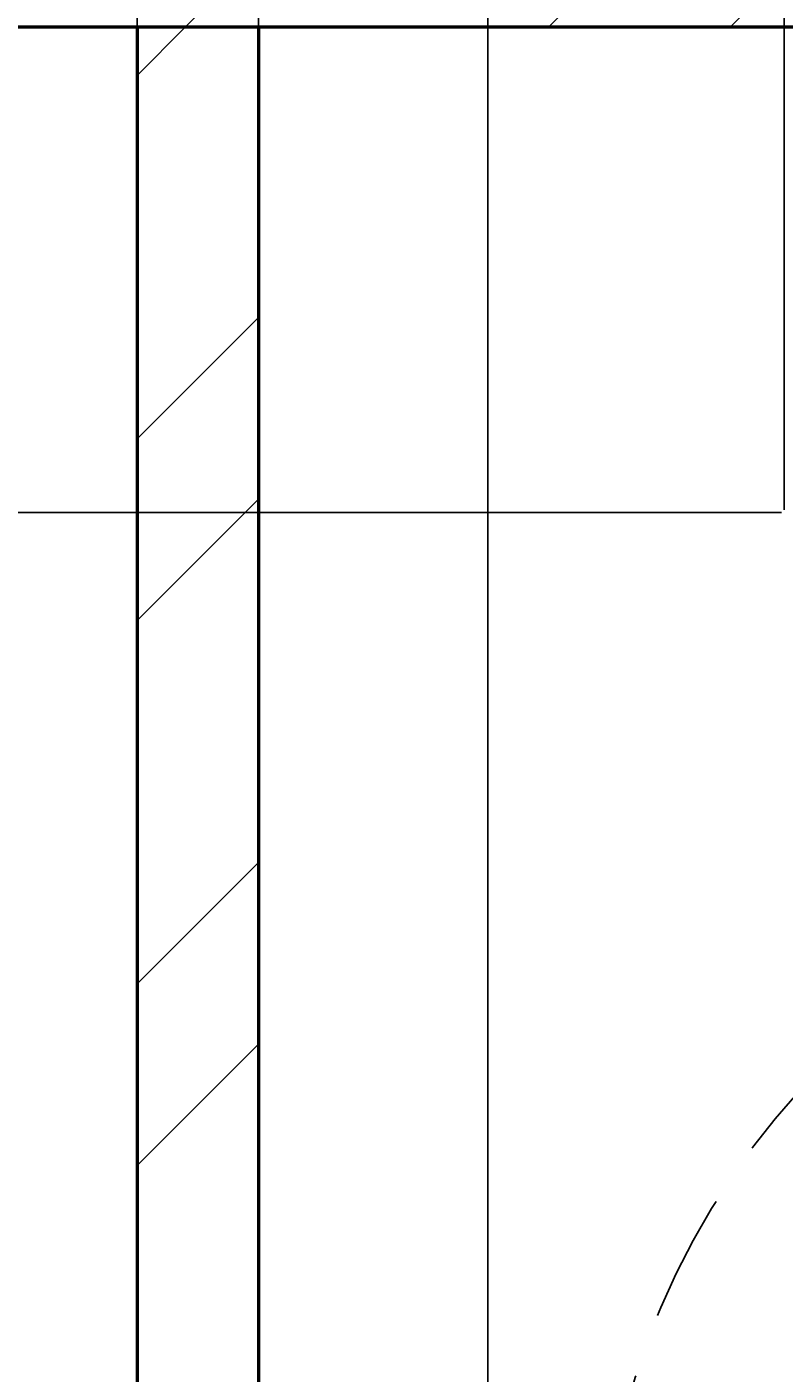
# Model space of a CAD drawing. Units: inches. Extents: x 2812 to 3051, y 1398 to 1659.
# Tile 53 of 65: x 2878 to 2896, y 1605 to 1638. Entities that reach past the tile are written whole.
import ezdxf

# ---------------------------------------------------------------- set-up
doc = ezdxf.new("R2010")
doc.units = ezdxf.units.IN
doc.linetypes.add('HIDDEN2', pattern=[4.7625, 3.175, -1.5875])
for name, color, linetype, lineweight in [('A-ANNO-DIMS', 2, 'Continuous', 18), ('S-CONC', 7, 'Continuous', 50), ('S-CONC-HIDN', 8, 'HIDDEN2', 25), ('S-CONC-PATT', 8, 'Continuous', 18)]:
    doc.layers.add(name, color=color, linetype=linetype, lineweight=lineweight)
doc.styles.get("Standard").update_dxf_attribs({"font": 'arial.ttf'})
doc.dimstyles.get("Standard").update_dxf_attribs({"dimtxt": 0.18, "dimasz": 0.18, "dimexe": 0.18, "dimexo": 0.0625, "dimgap": 0.09, "dimtad": 0, "dimtih": 1, "dimtoh": 1, "dimdec": 4, "dimzin": 0, "dimdsep": 46, "dimtxsty": 'Standard', "dimcen": 0.09, "dimadec": 0, "dimazin": 0, "dimtfac": 1, "dimtdec": 4, "dimtofl": 0, "dimtmove": 0, "dimatfit": 3, "dimfxl": 1, "dimtolj": 1, "dimtzin": 0, "dimarcsym": 0})

# ---------------------------------------------------------------- blocks, each defined once
blk = doc.blocks.new('*D17')
at = {"layer": 'A-ANNO-DIMS', "color": 0, "lineweight": -2, "transparency": 16777216}
for p, q in [((2883.385, 1637.882), (2883.385, 1659.35)), ((2896.385, 1625.882), (2896.385, 1659.35)), ((2883.565, 1659.17), (2889.674, 1659.17)), ((2896.205, 1659.17), (2890.095, 1659.17))]:
    blk.add_line(p, q, dxfattribs=at)
at = {"layer": 'A-ANNO-DIMS', "color": 0, "transparency": 16777216}
for points in [[(2883.565, 1659.2), (2883.565, 1659.14), (2883.385, 1659.17)], [(2896.205, 1659.2), (2896.205, 1659.14), (2896.385, 1659.17)]]:
    blk.add_solid(points, dxfattribs=at)
at = {"layer": 'Defpoints', "color": 0, "transparency": 16777216}
for p in [(2896.385, 1659.17), (2883.385, 1637.82), (2896.385, 1625.82)]:
    blk.add_point(p, dxfattribs=at)
at = {"layer": 'A-ANNO-DIMS', "color": 0, "transparency": 16777216, "insert": (2889.885, 1659.17), "char_height": 0.18, "attachment_point": 5}
blk.add_mtext('\\A1;13', dxfattribs=at)
blk = doc.blocks.new('*D18')
at = {"layer": 'A-ANNO-DIMS', "color": 0, "lineweight": -2, "transparency": 16777216}
for p, q in [((2896.385, 1625.882), (2896.385, 1659.35)), ((2905.385, 1625.882), (2905.385, 1659.35)), ((2896.565, 1659.17), (2900.736, 1659.17)), ((2905.205, 1659.17), (2901.034, 1659.17))]:
    blk.add_line(p, q, dxfattribs=at)
at = {"layer": 'A-ANNO-DIMS', "color": 0, "transparency": 16777216}
for points in [[(2896.565, 1659.2), (2896.565, 1659.14), (2896.385, 1659.17)], [(2905.205, 1659.2), (2905.205, 1659.14), (2905.385, 1659.17)]]:
    blk.add_solid(points, dxfattribs=at)
at = {"layer": 'Defpoints', "color": 0, "transparency": 16777216}
for p in [(2905.385, 1659.17), (2896.385, 1625.82), (2905.385, 1625.82)]:
    blk.add_point(p, dxfattribs=at)
at = {"layer": 'A-ANNO-DIMS', "color": 0, "transparency": 16777216, "insert": (2900.885, 1659.17), "char_height": 0.18, "attachment_point": 5}
blk.add_mtext('\\A1;9', dxfattribs=at)
blk = doc.blocks.new('*D38')
at = {"layer": 'A-ANNO-DIMS', "color": 0, "lineweight": -2, "transparency": 16777216}
for p, q in [((2896.322, 1625.82), (2811.806, 1625.82)), ((2811.986, 1625.64), (2811.986, 1612.5)), ((2811.986, 1599), (2811.986, 1612.14)), ((2910.679, 1598.82), (2811.806, 1598.82))]:
    blk.add_line(p, q, dxfattribs=at)
at = {"layer": 'A-ANNO-DIMS', "color": 0, "transparency": 16777216}
for points in [[(2811.956, 1625.64), (2812.016, 1625.64), (2811.986, 1625.82)], [(2811.956, 1599), (2812.016, 1599), (2811.986, 1598.82)]]:
    blk.add_solid(points, dxfattribs=at)
at = {"layer": 'Defpoints', "color": 0, "transparency": 16777216}
for p in [(2811.986, 1625.82), (2896.385, 1625.82), (2910.742, 1598.82)]:
    blk.add_point(p, dxfattribs=at)
at = {"layer": 'A-ANNO-DIMS', "color": 0, "transparency": 16777216, "insert": (2811.986, 1612.32), "char_height": 0.18, "attachment_point": 5}
blk.add_mtext('\\A1;27', dxfattribs=at)
blk = doc.blocks.new('*D39')
at = {"layer": 'A-ANNO-DIMS', "color": 0, "lineweight": -2, "transparency": 16777216}
for p, q in [((2883.322, 1637.82), (2811.806, 1637.82)), ((2811.986, 1637.64), (2811.986, 1632)), ((2811.986, 1626), (2811.986, 1631.64)), ((2896.322, 1625.82), (2811.806, 1625.82))]:
    blk.add_line(p, q, dxfattribs=at)
at = {"layer": 'A-ANNO-DIMS', "color": 0, "transparency": 16777216}
for points in [[(2811.956, 1637.64), (2812.016, 1637.64), (2811.986, 1637.82)], [(2811.956, 1626), (2812.016, 1626), (2811.986, 1625.82)]]:
    blk.add_solid(points, dxfattribs=at)
at = {"layer": 'Defpoints', "color": 0, "transparency": 16777216}
for p in [(2811.986, 1637.82), (2883.385, 1637.82), (2896.385, 1625.82)]:
    blk.add_point(p, dxfattribs=at)
at = {"layer": 'A-ANNO-DIMS', "color": 0, "transparency": 16777216, "insert": (2811.986, 1631.82), "char_height": 0.18, "attachment_point": 5}
blk.add_mtext('\\A1;12', dxfattribs=at)
blk = doc.blocks.new('*D58')
at = {"layer": 'A-ANNO-DIMS', "color": 0, "lineweight": -2, "transparency": 16777216}
for p, q in [((2880.385, 1472.098), (2880.385, 1659.35)), ((2883.385, 1472.098), (2883.385, 1659.35)), ((2880.565, 1659.17), (2881.736, 1659.17)), ((2883.205, 1659.17), (2882.034, 1659.17))]:
    blk.add_line(p, q, dxfattribs=at)
at = {"layer": 'A-ANNO-DIMS', "color": 0, "transparency": 16777216}
for points in [[(2880.565, 1659.2), (2880.565, 1659.14), (2880.385, 1659.17)], [(2883.205, 1659.2), (2883.205, 1659.14), (2883.385, 1659.17)]]:
    blk.add_solid(points, dxfattribs=at)
at = {"layer": 'Defpoints', "color": 0, "transparency": 16777216}
for p in [(2883.385, 1659.17), (2880.385, 1472.035), (2883.385, 1472.035)]:
    blk.add_point(p, dxfattribs=at)
at = {"layer": 'A-ANNO-DIMS', "color": 0, "transparency": 16777216, "insert": (2881.885, 1659.17), "char_height": 0.18, "attachment_point": 5}
blk.add_mtext('\\A1;3', dxfattribs=at)
blk = doc.blocks.new('*D59')
at = {"layer": 'A-ANNO-DIMS', "color": 0, "lineweight": -2, "transparency": 16777216}
for p, q in [((2883.385, 1452.098), (2883.385, 1659.35)), ((2889.058, 1467.465), (2889.058, 1659.35)), ((2883.565, 1659.17), (2885.828, 1659.17)), ((2888.878, 1659.17), (2886.615, 1659.17))]:
    blk.add_line(p, q, dxfattribs=at)
at = {"layer": 'A-ANNO-DIMS', "color": 0, "transparency": 16777216}
for points in [[(2883.565, 1659.2), (2883.565, 1659.14), (2883.385, 1659.17)], [(2888.878, 1659.2), (2888.878, 1659.14), (2889.058, 1659.17)]]:
    blk.add_solid(points, dxfattribs=at)
at = {"layer": 'Defpoints', "color": 0, "transparency": 16777216}
for p in [(2889.058, 1659.17), (2889.058, 1467.402), (2883.385, 1452.035)]:
    blk.add_point(p, dxfattribs=at)
at = {"layer": 'A-ANNO-DIMS', "color": 0, "transparency": 16777216, "insert": (2886.221, 1659.17), "char_height": 0.18, "attachment_point": 5}
blk.add_mtext('\\A1;5.673', dxfattribs=at)

msp = doc.modelspace()

# ---------------------------------------------------------------- hatches: boundary and pattern name
at = {"layer": 'S-CONC-PATT'}
h = msp.add_hatch(dxfattribs=at)
h.set_pattern_fill('ANSI32', color=256)
h.paths.add_polyline_path([(3027.3849, 1646.82), (2835.3849, 1646.82), (2835.3849, 1603.2296), (2844.3849, 1603.2296), (2844.3849, 1637.82), (3018.3849, 1637.82), (3018.3849, 1602.5441), (3027.3849, 1602.5441)])
h.paths.add_polyline_path([(2844.3849, 1594.2296), (2835.3849, 1594.2296), (2835.3849, 1550.82), (3027.3849, 1550.82), (3027.3849, 1593.5441), (3018.3849, 1593.5441), (3018.3849, 1559.82), (2844.3849, 1559.82)])
h.paths.add_polyline_path([(2844.3849, 1482.0354), (2835.3849, 1482.0354), (2835.3849, 1463.4959), (2844.3849, 1463.4959)])
h.paths.add_polyline_path([(2844.3849, 1461.4959), (2835.3849, 1461.4959), (2835.3849, 1416.0354), (2844.3849, 1416.0354)])
h.paths.add_polyline_path([(3027.3849, 1482.0354), (3018.3849, 1482.0354), (3018.3849, 1463.2854), (3027.3849, 1463.2854)])
h.paths.add_polyline_path([(3027.3849, 1461.2854), (3018.3849, 1461.2854), (3018.3849, 1416.0354), (3027.3849, 1416.0354)])
h.paths.add_polyline_path([(2961.3849, 1448.4738), (2952.3849, 1448.4738), (2952.3849, 1416.0354), (2961.3849, 1416.0354)])
h.paths.add_polyline_path([(2961.3849, 1462.3026), (2952.3849, 1462.3026), (2952.3849, 1450.4738), (2961.3849, 1450.4738)])
h.paths.add_polyline_path([(2961.3849, 1472.0354), (2952.3849, 1472.0354), (2952.3849, 1462.3026), (2961.3849, 1462.3026)])
h = msp.add_hatch(dxfattribs=at)
h.set_pattern_fill('ANSI32', color=256)
h.paths.add_polyline_path([(2961.3849, 1637.82), (2952.3849, 1637.82), (2952.3849, 1603.2541), (2961.3849, 1603.2541)])
h.paths.add_polyline_path([(2961.3849, 1594.2541), (2952.3849, 1594.2541), (2952.3849, 1559.82), (2961.3849, 1559.82)])
h.paths.add_polyline_path([(2883.3849, 1637.82), (2880.3849, 1637.82), (2880.3849, 1559.82), (2883.3849, 1559.82)])

# ---------------------------------------------------------------- linework, layer by layer
at = {"layer": 'S-CONC'}
for p, q in [((2844.3849, 1637.82), (3018.3849, 1637.82)), ((2880.3849, 1637.82), (2880.3849, 1559.82)), ((2883.3849, 1637.82), (2883.3849, 1559.82))]:
    msp.add_line(p, q, dxfattribs=at)
at = {"layer": 'S-CONC-HIDN'}
msp.add_circle((2910.7415, 1598.82), 18.8884, dxfattribs=at)

# ---------------------------------------------------------------- dimensions: what is measured, and where the dimension line sits
at = {"layer": 'A-ANNO-DIMS'}
for base, p1, p2, override, picture, middle in [((2883.3849, 1659.17), (2880.3849, 1472.0354), (2883.3849, 1472.0354), {"dimdec": 0, "dimlfac": 1, "dimrnd": 0, "dimzin": 0, "dimdsep": 46, "dimlunit": 2}, '*D58', (2881.8849, 1659.17)), ((2896.3849, 1659.17), (2883.3849, 1637.82), (2896.3849, 1625.82), {"dimdec": 0, "dimlfac": 1, "dimrnd": 0, "dimzin": 0, "dimdsep": 46, "dimlunit": 2}, '*D17', (2889.8849, 1659.17)), ((2889.0577, 1659.17), (2883.3849, 1452.0354), (2889.0577, 1467.4024), {"dimdec": 3, "dimlfac": 1, "dimrnd": 0, "dimzin": 0, "dimdsep": 46, "dimlunit": 2}, '*D59', (2886.2213, 1659.17)), ((2905.3849, 1659.17), (2896.3849, 1625.82), (2905.3849, 1625.82), {"dimdec": 0, "dimlfac": 1, "dimrnd": 0, "dimzin": 0, "dimdsep": 46, "dimlunit": 2}, '*D18', (2900.8849, 1659.17))]:
    dim = msp.add_linear_dim(base=base, p1=p1, p2=p2, dimstyle='Standard', override=override, dxfattribs=at)
    dim.commit()
    dim.dimension.update_dxf_attribs({"geometry": picture, "text_midpoint": middle})
for base, p1, p2, picture, middle in [((2811.9855, 1637.82), (2896.3849, 1625.82), (2883.3849, 1637.82), '*D39', (2811.9855, 1631.82)), ((2811.9855, 1625.82), (2910.7415, 1598.82), (2896.3849, 1625.82), '*D38', (2811.9855, 1612.32))]:
    dim = msp.add_linear_dim(base=base, p1=p1, p2=p2, angle=90, dimstyle='Standard', override={"dimdec": 0, "dimlfac": 1, "dimrnd": 0, "dimzin": 0, "dimdsep": 46, "dimlunit": 2}, dxfattribs=at)
    dim.commit()
    dim.dimension.update_dxf_attribs({"geometry": picture, "text_midpoint": middle})

doc.saveas('drawing.dxf')
